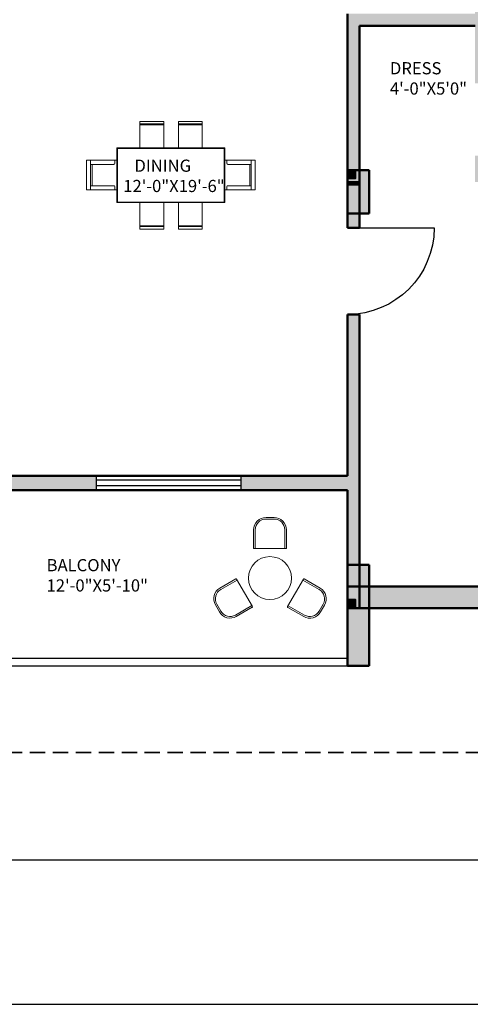
# Model space of a CAD drawing. Units: inches. Extents: x -7 to 1228, y -146 to 1091.
# Tile 34 of 88: x 815 to 1002, y -105 to 304. Entities that reach past the tile are written whole.
import ezdxf

# ---------------------------------------------------------------- set-up
doc = ezdxf.new("R2010")
doc.units = ezdxf.units.IN
doc.linetypes.add('DASHED2', pattern=[9.525, 6.35, -3.175])
for name, color, linetype, lineweight in [('A-AREA-IDEN', 7, 'Continuous', 18), ('A-COLS', 6, 'Continuous', 35), ('A-DOOR', 4, 'Continuous', 25), ('A-FURN', 8, 'Continuous', 18), ('A-GLAZ', 175, 'Continuous', 25), ('A-WALL', 7, 'Continuous', 50), ('A-WALL-PATT', 251, 'Continuous', 13), ('C-PROP', 1, 'DASHED2', 35), ('C-ROAD', 7, 'Continuous', 25)]:
    doc.layers.add(name, color=color, linetype=linetype, lineweight=lineweight)
doc.styles.get("Standard").update_dxf_attribs({"font": 'arial.ttf'})

# ---------------------------------------------------------------- blocks, each defined once
blk = doc.blocks.new('A$C317A697B')
for p, q in [((-116, 441), (-514, 441)), ((-514, 441), (-514, 0)), ((-116, 398), (-514, 398)), ((-116, 385), (-514, 385)), ((-116, 0), (-116, 441)), ((523, 441), (125, 441)), ((125, 441), (125, 0)), ((523, 398), (125, 398)), ((523, 385), (125, 385)), ((523, 0), (523, 441)), ((-899, -912), (-899, 0)), ((-899, 0), (899, 0)), ((899, 0), (899, -912)), ((-889, -902), (-889, -10)), ((-889, -10), (889, -10)), ((889, -10), (889, -902)), ((-899, -205), (-1402, -205)), ((-1402, -205), (-1402, -699)), ((-1336, -205), (-1336, -699)), ((-946, -274), (-1336, -274)), ((-1311, -274), (-1311, -630)), ((-932, -205), (-932, -259)), ((899, -205), (1402, -205)), ((932, -205), (932, -259)), ((946, -274), (1336, -274)), ((1311, -274), (1311, -630)), ((1336, -205), (1336, -699)), ((1402, -205), (1402, -699)), ((-946, -630), (-1336, -630)), ((-932, -699), (-932, -645)), ((932, -699), (932, -645)), ((946, -630), (1336, -630)), ((-1402, -699), (-899, -699)), ((1402, -699), (899, -699)), ((899, -912), (-899, -912)), ((889, -902), (-889, -902)), ((-514, -1353), (-514, -912)), ((-116, -912), (-116, -1353)), ((125, -1353), (125, -912)), ((523, -912), (523, -1353)), ((-116, -1297), (-514, -1297)), ((-116, -1309), (-514, -1309)), ((523, -1297), (125, -1297)), ((523, -1309), (125, -1309)), ((-116, -1353), (-514, -1353)), ((523, -1353), (125, -1353))]:
    blk.add_line(p, q)
for centre, start, end in [((-946, -259), 270, 0), ((946, -259), 180, 270), ((-946, -645), 0, 90), ((946, -645), 90, 180)]:
    blk.add_arc(centre, 14.7, start, end)
blk = doc.blocks.new('A$C670C3AF2')
for p, q in [((1122, 1874), (972, 1874)), ((1122, 1844), (972, 1844)), ((742, 1644), (742, 1304)), ((772, 1644), (772, 1294)), ((1322, 1294), (1322, 1644)), ((1352, 1304), (1352, 1644)), ((752, 1294), (1342, 1294)), ((409, 730), (115, 560)), ((433, 709), (130, 534)), ((718, 215), (423, 726)), ((1669, 725), (1374, 214)), ((1963, 533), (1659, 708)), ((1978, 559), (1683, 729)), ((30, 246), (105, 116)), ((56, 261), (131, 131)), ((405, 58), (708, 233)), ((420, 32), (714, 202)), ((1378, 200), (1673, 30)), ((1384, 231), (1688, 56)), ((1961, 130), (2036, 259)), ((1987, 115), (2062, 244))]:
    blk.add_line(p, q)
blk.add_circle((1046, 745), 400)
for centre, radius, start, end in [((972, 1644), 230, 90, 180), ((972, 1644), 200, 90, 180), ((1122, 1644), 230, 0, 90), ((1122, 1644), 200, 0, 90), ((752, 1304), 10, 180, 270), ((1342, 1304), 10, 270, 0), ((230, 361), 230, 120, 210), ((414, 721), 10, 30, 120), ((1678, 720), 10, 60, 150), ((1863, 359), 230, 330, 60), ((230, 361), 200, 120, 210), ((1863, 359), 200, 330, 60), ((709, 210), 10, 300, 30), ((1383, 209), 10, 150, 240), ((305, 231), 230, 210, 300), ((305, 231), 200, 210, 300), ((1788, 230), 230, 240, 330), ((1788, 230), 200, 240, 330)]:
    blk.add_arc(centre, radius, start, end)
blk = doc.blocks.new('WIN-BALCONY-60')
for p, q in [((0, 0), (0, 6)), ((0, 6), (60, 6)), ((0, 4.29), (60, 4.29)), ((60, 6), (60, 0)), ((60, 4.29), (60, 1.76)), ((60, 1.76), (0, 1.76)), ((60, 0), (0, 0))]:
    blk.add_line(p, q)
blk = doc.blocks.new('DOOR-900')
blk.add_line((36, 0), (36, 36))
blk.add_arc((36, 0), 36, 90, 180)

msp = doc.modelspace()

# ---------------------------------------------------------------- hatches: boundary and pattern name
at = {"layer": 'A-COLS'}
h = msp.add_hatch(color=256, dxfattribs=at)
h.dxf.hatch_style = 1
h.paths.add_polyline_path([(960, 224), (951, 224), (951, 238.45), (954.29, 238.45), (954.29, 242), (960, 242)])
h = msp.add_hatch(color=256, dxfattribs=at)
h.dxf.hatch_style = 1
h.paths.add_polyline_path([(954.29, 238.45), (954.29, 242), (951, 242), (951, 238.45)])
h = msp.add_hatch(color=256, dxfattribs=at)
h.dxf.hatch_style = 1
h.paths.add_polyline_path([(951, 63.55), (954.29, 63.55), (954.29, 60), (960, 60), (960, 78), (951, 78)])
h = msp.add_hatch(color=256, dxfattribs=at)
h.dxf.hatch_style = 1
h.paths.add_polyline_path([(951, 63.55), (951, 60), (954.29, 60), (954.29, 63.55)])
at = {"layer": 'A-WALL-PATT'}
h = msp.add_hatch(color=256, dxfattribs=at)
h.dxf.hatch_style = 1
h.paths.add_polyline_path([(69, 568), (60, 568), (60, 493), (63.29, 493), (69, 493)])
h.paths.add_polyline_path([(69, 662.41), (60, 662.41), (60, 586), (69, 586)], flags=17)
h.paths.add_polyline_path([(69, 723), (184, 723), (184, 734), (179, 734), (179, 728), (69, 728), (69, 741.62), (60, 741.62), (60, 698.41), (69, 698.41)], flags=17)
h.paths.add_polyline_path([(69, 782), (231, 782), (231, 728), (231, 723), (231, 586), (236, 586), (236, 787), (69, 787), (69, 800.13), (60, 800.13), (60, 765.62), (69, 765.62)])
h.paths.add_polyline_path([(184, 842), (189, 842), (189, 848), (173, 848), (173, 842), (179, 842), (179, 787), (184, 787)])
h.paths.add_polyline_path([(118.22, 69), (69, 69), (69, 60), (118.22, 60)])
h.paths.add_polyline_path([(227, 69), (154.22, 69), (154.22, 60), (227, 60)])
h.paths.add_polyline_path([(236, 60), (232.71, 60), (227, 60), (227, 36), (236, 36)])
h.paths.add_polyline_path([(389, 60), (380, 60), (380, 36), (389, 36)])
h.paths.add_polyline_path([(384, 181), (380, 181), (380, 115), (380, 78), (384, 78)])
h.paths.add_polyline_path([(380, 115), (334.55, 115), (334.55, 109), (380, 109)])
h.paths.add_polyline_path([(274.55, 115), (236, 115), (236, 201), (232.71, 201), (231, 201), (231, 78), (236, 78), (236, 109), (274.55, 109)])
h.paths.add_polyline_path([(69, 123), (60, 123), (60, 78), (69, 78)])
h.paths.add_polyline_path([(69, 201), (60, 201), (60, 159), (69, 159)])
h.paths.add_polyline_path([(143, 219), (69, 219), (69, 213), (143, 213)], flags=17)
h.paths.add_polyline_path([(189, 219), (184, 219), (184, 274), (231, 274), (231, 219), (236, 219), (236, 279), (184, 279), (184, 297), (179, 297), (179, 279), (69, 279), (69, 290.91), (60, 290.91), (60, 262.18), (69, 262.18), (69, 274), (179, 274), (179, 219), (173, 219), (173, 213), (189, 213)])
h.paths.add_polyline_path([(69, 238.18), (60, 238.18), (60, 219), (69, 219)], flags=17)
h.paths.add_polyline_path([(69, 333), (60, 333), (60, 314.91), (69, 314.91), (69, 316.96)])
h.paths.add_polyline_path([(190, 338), (184, 338), (69, 338), (69, 333), (179, 333), (179, 327), (184, 327), (184, 333.02), (190, 333.05)])
h.paths.add_polyline_path([(69, 386.81), (60, 386.81), (60, 351), (69, 351)])
h.paths.add_polyline_path([(69, 475), (60, 475), (60, 422.81), (69, 422.81)])
h.paths.add_polyline_path([(236, 475), (231, 475), (231, 351.24), (236, 351.24)])
h.paths.add_polyline_path([(384, 475), (380, 475), (380, 362), (384, 362)])
h.paths.add_polyline_path([(547, 307), (439, 307), (439, 356), (445, 356), (445, 362), (433, 362), (433, 307), (380, 307), (380, 244), (380, 241), (384, 241), (384, 301), (433, 301), (433, 277), (439, 277), (439, 301), (547, 301)])
h.paths.add_polyline_path([(547, 241), (439, 241), (439, 247), (433, 247), (433, 235), (547, 235)])
h.paths.add_polyline_path([(450, 69), (440.29, 69), (424.89, 69), (389, 69), (389, 60), (450, 60)])
h.paths.add_polyline_path([(547, 69), (486, 69), (486, 60), (547, 60)])
h.paths.add_polyline_path([(556, 148.27), (547, 148.27), (547, 78), (556, 78)])
h.paths.add_polyline_path([(556, 223), (547, 223), (547, 195), (547, 184.27), (556, 184.27)])
h.paths.add_polyline_path([(556, 311.19), (547, 311.19), (547, 273.08), (556, 273.08)])
h.paths.add_polyline_path([(556, 344), (552.71, 344), (547, 344), (547, 335.19), (556, 335.19)])
h.paths.add_polyline_path([(556, 249.08), (547, 249.08), (547, 241), (556, 241)])
h.paths.add_polyline_path([(547, 362), (475, 362), (475, 356), (547, 356)], flags=0)
h.paths.add_polyline_path([(556, 399.62), (547, 399.62), (547, 362), (556, 362)])
h.paths.add_polyline_path([(556, 475), (547, 475), (547, 435.62), (556, 435.62)])
h.paths.add_polyline_path([(547, 493), (389, 493), (389, 487), (547, 487)])
h.paths.add_polyline_path([(380, 493), (278, 493), (278, 487), (380, 487)])
h.paths.add_polyline_path([(227, 493), (69, 493), (69, 487), (227, 487)])
h.paths.add_polyline_path([(643, 122.44), (634, 122.44), (634, 78), (643, 78)])
h.paths.add_polyline_path([(702.5, 69), (692.79, 69), (677.39, 69), (643, 69), (643, 60), (702.5, 60)])
h.paths.add_polyline_path([(798, 69), (738.5, 69), (738.5, 60), (798, 60)])
h.paths.add_polyline_path([(807, 60), (803.71, 60), (798, 60), (798, 36), (807, 36)])
h.paths.add_polyline_path([(807, 109), (846.75, 109), (846.75, 115), (807, 115), (807, 159), (802, 159), (802, 78), (807, 78)])
h.paths.add_polyline_path([(807, 201), (802, 201), (802, 195), (807, 195)])
h.paths.add_polyline_path([(643, 201), (634, 201), (634, 158.44), (643, 158.44)])
h.paths.add_polyline_path([(756, 225), (751, 225), (751, 219), (643, 219), (643, 213), (756, 213)])
h.paths.add_polyline_path([(643, 240.85), (634, 240.85), (634, 219), (643, 219)])
h.paths.add_polyline_path([(643, 274), (643, 288.63), (634, 288.63), (634, 264.85), (643, 264.85)])
h.paths.add_polyline_path([(802, 279), (756, 279), (756, 297), (751, 297), (751, 279), (643, 279), (643, 274), (751, 274), (751, 255), (756, 255), (756, 274), (802, 274)])
h.paths.add_polyline_path([(807, 333), (803.71, 333), (802, 333), (802, 279), (802, 274), (802, 219), (807, 219)])
h.paths.add_polyline_path([(956, 182), (951, 182), (951, 115), (906.75, 115), (906.75, 109), (951, 109), (951, 78), (956, 78)])
h.paths.add_polyline_path([(960, 60), (951, 60), (951, 36), (960, 36)])
h.paths.add_polyline_path([(1021, 69), (1005.78, 69), (960, 69), (960, 60), (1021, 60)])
h.paths.add_polyline_path([(956, 224), (951, 224), (951, 218), (956, 218)])
h.paths.add_polyline_path([(956, 302), (1004, 302), (1004, 278), (1010, 278), (1010, 302), (1118, 302), (1118, 290.81), (1127, 290.81), (1127, 326.97), (1118, 326.97), (1118, 320.97), (1118, 307), (1010, 307), (1010, 356), (1016, 356), (1016, 362), (1004, 362), (1004, 307), (951, 307), (951, 244), (951, 242), (954.29, 242), (956, 242)])
h.paths.add_polyline_path([(643, 333), (634, 333), (634, 312.63), (643, 312.63), (643, 316.96)])
h.paths.add_polyline_path([(756, 338), (643, 338), (643, 333), (751, 333), (751, 327), (756, 327)])
h.paths.add_polyline_path([(643, 388), (634, 388), (634, 351), (643, 351)])
h.paths.add_polyline_path([(807, 357), (802, 357), (802, 351), (807, 351)])
h.paths.add_polyline_path([(807, 475), (802, 475), (802, 393), (807, 393)])
h.paths.add_polyline_path([(643, 475), (634, 475), (634, 424), (643, 424)])
h.paths.add_polyline_path([(798, 493), (643, 493), (643, 487), (798, 487)])
h.paths.add_polyline_path([(634, 493), (556, 493), (556, 487), (634, 487)])
h.paths.add_polyline_path([(813, 493), (807, 493), (807, 487), (813, 487)])
h.paths.add_polyline_path([(951, 493), (849, 493), (849, 487), (951, 487)])
h.paths.add_polyline_path([(956, 484), (951, 484), (951, 374), (956, 374)])
h.paths.add_polyline_path([(1109, 493), (969, 493), (969, 487), (1109, 487)])
h.paths.add_polyline_path([(1127, 484), (1118, 484), (1118, 450.64), (1127, 450.64)])
h.paths.add_polyline_path([(1127, 414.64), (1118, 414.64), (1118, 365), (1127, 365)])
h.paths.add_polyline_path([(1109, 362), (1046, 362), (1046, 356), (1109, 356)], flags=17)
h.paths.add_polyline_path([(1127, 356), (1123.45, 356), (1118, 356), (1118, 350.97), (1127, 350.97)], flags=0)
h.paths.add_polyline_path([(1127, 266.81), (1118, 266.81), (1118, 262.36), (1118, 242), (1127, 242)], flags=17)
h.paths.add_polyline_path([(1118, 242), (1010, 242), (1010, 248), (1004, 248), (1004, 237), (1118, 237)])
h.paths.add_polyline_path([(1127, 224), (1118, 224), (1118, 170), (1127, 170)])
h.paths.add_polyline_path([(1127, 134), (1118, 134), (1118, 78), (1127, 78)])
h.paths.add_polyline_path([(1118, 69), (1057, 69), (1057, 60), (1118, 60)])
h.paths.add_polyline_path([(227, 571.55), (227, 574), (69, 574), (69, 568), (227, 568)])
h.paths.add_polyline_path([(380, 571.55), (380, 574), (278, 574), (278, 568), (380, 568)])
h.paths.add_polyline_path([(242, 574), (236, 574), (236, 568), (242, 568)])
h.paths.add_polyline_path([(547, 571.55), (547, 574), (389, 574), (389, 568), (547, 568)])
h.paths.add_polyline_path([(384, 733), (380, 733), (380, 586), (384, 586)])
h.paths.add_polyline_path([(556, 646), (634, 646), (634, 655), (547, 655), (547, 586), (556, 586)])
h.paths.add_polyline_path([(634, 574), (556, 574), (556, 568), (634, 568)])
h.paths.add_polyline_path([(643, 655), (634, 655), (634, 586), (643, 586)])
h.paths.add_polyline_path([(798, 574), (643, 574), (643, 568), (798, 568)])
h.paths.add_polyline_path([(643, 663.85), (634, 663.85), (634, 655), (643, 655)])
h.paths.add_polyline_path([(556, 676.97), (547, 676.97), (547, 655), (556, 655)])
h.paths.add_polyline_path([(556, 733), (547, 733), (547, 712.97), (556, 712.97)])
h.paths.add_polyline_path([(643, 710), (634, 710), (634, 699.85), (643, 699.85)])
h.paths.add_polyline_path([(807, 668), (802, 668), (802, 586), (807, 586)])
h.paths.add_polyline_path([(951, 574), (849, 574), (849, 568), (951, 568)])
h.paths.add_polyline_path([(956, 691), (951, 691), (951, 577), (956, 577)])
h.paths.add_polyline_path([(1109, 574), (969, 574), (969, 568), (1109, 568)])
h.paths.add_polyline_path([(1127, 643.4), (1118, 643.4), (1118, 577), (1127, 577)])
h.paths.add_polyline_path([(1127, 568), (1123.45, 568), (1118, 568), (1118, 493), (1127, 493)])
h.paths.add_polyline_path([(1127, 733), (1118, 733), (1118, 679.4), (1127, 679.4)])
h.paths.add_polyline_path([(1127, 777.35), (1118, 777.35), (1118, 770.04), (1118, 751), (1127, 751)], flags=17)
h.paths.add_polyline_path([(1118, 751), (1010, 751), (1010, 757), (1004, 757), (1004, 745), (1118, 745)])
h.paths.add_polyline_path([(956, 811), (1004, 811), (1004, 787), (1010, 787), (1010, 811), (1017.87, 811), (1017.87, 811.63, -0.414214), (1018.25, 812), (1031.98, 812, -0.414214), (1032.35, 811.63), (1032.35, 811), (1118, 811), (1118, 801.35), (1127, 801.35), (1127, 834.69), (1118, 834.69), (1118, 830.24), (1118, 817), (1010, 817), (1010, 866), (1016, 866), (1016, 872), (1004, 872), (1004, 817), (956, 817), (956, 866), (951, 866), (951, 751), (954.29, 751), (956, 751)])
h.paths.add_polyline_path([(1118, 872), (1046, 872), (1046, 866), (1118, 866)], flags=17)
h.paths.add_polyline_path([(1127, 924.71), (1118, 924.71), (1118, 884), (1127, 884)])
h.paths.add_polyline_path([(1127, 866), (1123.71, 866), (1118, 866), (1118, 858.69), (1127, 858.69)], flags=17)
h.paths.add_polyline_path([(956, 983), (951, 983), (951, 952), (807, 952), (807, 983), (802, 983), (802, 902), (807, 902), (807, 946), (951, 946), (951, 884), (956, 884)])
h.paths.add_polyline_path([(807, 842), (802, 842), (802, 787), (756, 787), (756, 806), (751, 806), (751, 787), (643, 787), (643, 782), (751, 782), (751, 764), (756, 764), (756, 782), (802, 782), (802, 728), (807, 728)])
h.paths.add_polyline_path([(756, 848), (643, 848), (643, 842), (751, 842), (751, 836), (756, 836)])
h.paths.add_polyline_path([(756, 734), (751, 734), (751, 728), (643, 728), (643, 723), (756, 723)])
h.paths.add_polyline_path([(643, 749.79), (634, 749.79), (634, 728), (637.29, 728), (643, 728)])
h.paths.add_polyline_path([(643, 805.41), (634, 805.41), (634, 773.79), (643, 773.79)])
h.paths.add_polyline_path([(643, 896.66), (634, 896.66), (634, 860), (637.29, 860), (643, 860)])
h.paths.add_polyline_path([(643, 842), (634, 842), (634, 829.41), (643, 829.41)])
h.paths.add_polyline_path([(643, 983), (634, 983), (634, 932.66), (643, 932.66)])
h.paths.add_polyline_path([(1127, 983), (1118, 983), (1118, 960.71), (1127, 960.71)])
h.paths.add_polyline_path([(1118, 1001), (1077.53, 1001), (1077.53, 992), (1118, 992)])
h.paths.add_polyline_path([(1041.53, 1001), (960, 1001), (960, 992), (1041.53, 992)])
h.paths.add_polyline_path([(960, 1025), (951, 1025), (951, 1001), (954.29, 1001), (960, 1001)])
h.paths.add_polyline_path([(807, 1025), (798, 1025), (798, 1001), (807, 1001)])
h.paths.add_polyline_path([(798, 1001), (738.5, 1001), (738.5, 992), (798, 992)])
h.paths.add_polyline_path([(702.5, 1001), (643, 1001), (643, 992), (702.5, 992)])
h.paths.add_polyline_path([(547, 1001), (499.11, 1001), (499.11, 992), (547, 992)])
h.paths.add_polyline_path([(463.11, 1001), (389, 1001), (389, 992), (463.11, 992)])
h.paths.add_polyline_path([(389, 1025), (380, 1025), (380, 1022), (380, 1001), (383.29, 1001), (389, 1001)])
h.paths.add_polyline_path([(236, 1025), (227, 1025), (227, 1001), (236, 1001)])
h.paths.add_polyline_path([(236, 983), (231, 983), (231, 860), (236, 860)])
h.paths.add_polyline_path([(274.55, 952), (236, 952), (236, 946), (274.55, 946)])
h.paths.add_polyline_path([(380, 952), (334.55, 952), (334.55, 946), (380, 946)])
h.paths.add_polyline_path([(384, 983), (380, 983), (380, 884), (383.29, 884), (384, 884)])
h.paths.add_polyline_path([(227, 1001), (155.01, 1001), (155.01, 992), (162.87, 992), (227, 992)])
h.paths.add_polyline_path([(119.01, 1001), (69, 1001), (69, 992), (119.01, 992)])
h.paths.add_polyline_path([(69, 983), (60, 983), (60, 922.99), (69, 922.99)])
h.paths.add_polyline_path([(69, 886.99), (60, 886.99), (60, 860), (63.29, 860), (69, 860)])
h.paths.add_polyline_path([(143, 848), (69, 848), (69, 842), (143, 842)])

# ---------------------------------------------------------------- linework, layer by layer
at = {"layer": 'A-COLS'}
for points in [[(951, 242), (954.29, 242), (954.29, 238.45), (951, 238.45)], [(951, 60), (954.29, 60), (954.29, 63.55), (951, 63.55)]]:
    msp.add_lwpolyline(points, close=True, dxfattribs=at)
at = {"layer": 'A-GLAZ'}
for p, q in [((951, 39), (807, 39)), ((807, 36), (951, 36))]:
    msp.add_line(p, q, dxfattribs=at)
at = {"layer": 'A-WALL'}
for p, q in [((951, 244), (951, 307)), ((951, 307), (951, 218)), ((956, 250), (956, 302)), ((956, 302), (956, 218)), ((1004, 302), (956, 302)), ((956, 242), (951, 242)), ((951, 242), (960, 242)), ((951, 238.45), (951, 242)), ((956, 242), (951, 242)), ((960, 242), (960, 224)), ((956, 237), (951, 237)), ((956, 236), (951, 236)), ((951, 224), (951, 236)), ((960, 224), (951, 224)), ((956, 224), (951, 224)), ((956, 218), (951, 218)), ((951, 115), (951, 182)), ((956, 182), (951, 182)), ((951, 182), (951, 115)), ((956, 60), (956, 182)), ((956, 182), (956, 60)), ((951, 115), (807, 115)), ((951, 109), (807, 109)), ((951, 60), (951, 109)), ((951, 109), (951, 60)), ((960, 78), (951, 78)), ((951, 78), (951, 60)), ((960, 60), (960, 78)), ((1127, 69), (951, 69)), ((1127, 60), (951, 60)), ((951, 60), (951, 36)), ((951, 60), (960, 60)), ((951, 60), (1127, 60)), ((960, 36), (960, 60)), ((951, 36), (960, 36))]:
    msp.add_line(p, q, dxfattribs=at)
at = {"layer": 'C-PROP'}
msp.add_line((0, 0), (1187, 0), dxfattribs=at)
at = {"layer": 'C-ROAD'}
for p, q in [((0, -44.69), (1187, -44.69)), ((0, -104.69), (1187, -104.69))]:
    msp.add_line(p, q, dxfattribs=at)

# ---------------------------------------------------------------- block references
at = {"layer": 'A-DOOR', "extrusion": (0, 0, -1), "zscale": -1, "rotation": 89.99999999999989}
msp.add_blockref('DOOR-900', (-951, 182), dxfattribs=at)
at = {"layer": 'A-FURN'}
for name, p, xscale, yscale, zscale in [('A$C317A697B', (877.66, 251.23), 0.024965713951469, 0.024965713951469, 0.024965713951469), ('A$C670C3AF2', (895.47, 55.79), 0.022327308386288, 0.022327308386288, 0.022327308386288)]:
    msp.add_blockref(name, p, dxfattribs=dict(at, xscale=xscale, yscale=yscale, zscale=zscale))
at = {"layer": 'A-GLAZ', "rotation": 359.964472723119}
msp.add_blockref('WIN-BALCONY-60', (846.75, 109), dxfattribs=at)

# ---------------------------------------------------------------- texts
at = {"layer": 'A-AREA-IDEN', "attachment_point": 1}
for s, insert, char_height in [('DRESS\\P4\'-0"X5\'0"', (968.62, 286.85), 5.057), ('   DINING\\P12\'-0"X19\'-6"', (857.9, 246.35), 5.0568), ('BALCONY\\P12\'-0"X5\'-10"', (826.06, 80.34), 5.0568)]:
    msp.add_mtext_dynamic_manual_height_columns(s, width=137.2821, gutter_width=25.28, heights=[0], dxfattribs=dict(at, insert=insert, char_height=char_height))

doc.saveas('drawing.dxf')
